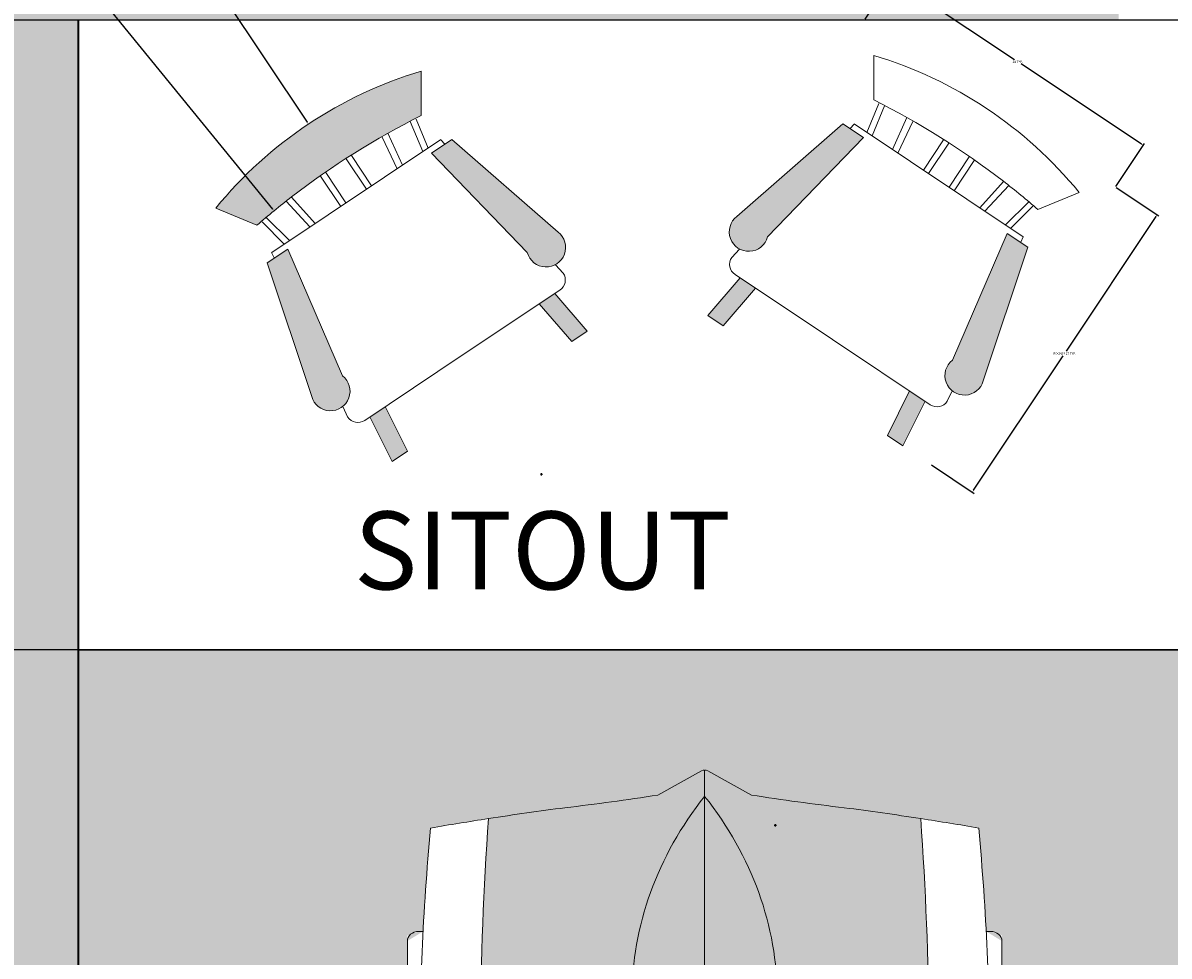
# Model space of a CAD drawing. Units: inches. Extents: x 2549 to 3108, y 1683 to 2362.
# Tile 5 of 30: x 2877 to 2970, y 1861 to 1936. Entities that reach past the tile are written whole.
import ezdxf

# ---------------------------------------------------------------- set-up
doc = ezdxf.new("R2010")
doc.units = ezdxf.units.IN
for name, color, linetype, lineweight in [('A-ANNO-DIMS', 2, 'Continuous', 18), ('A-AREA-IDEN', 7, 'Continuous', 18), ('A-FLOR', 7, 'Continuous', 25), ('A-FURN', 8, 'Continuous', 18), ('A-FURN-PATT', 9, 'Continuous', 13), ('A-WALL', 7, 'Continuous', 35), ('A-WALL-PATT', 89, 'Continuous', 13), ('C-PKNG-VEHI', 8, 'Continuous', 18)]:
    doc.layers.add(name, color=color, linetype=linetype, lineweight=lineweight)
doc.layers.add('C-PKNG-VEHI-PATT', color=251, linetype='Continuous', lineweight=13, true_color=0x636466)
doc.layers.add('C-PVMT-PATT', color=9, linetype='Continuous', lineweight=13, true_color=0xc7c8ca)
doc.styles.get("Standard").update_dxf_attribs({"font": 'arial.ttf'})
doc.dimstyles.get("Standard").update_dxf_attribs({"dimtxt": 0.18, "dimasz": 0.18, "dimexe": 0.18, "dimexo": 0.0625, "dimgap": 0.09, "dimtad": 0, "dimtih": 1, "dimtoh": 1, "dimdec": 4, "dimzin": 0, "dimdsep": 46, "dimtxsty": 'Standard', "dimcen": 0.09, "dimadec": 0, "dimazin": 0, "dimtfac": 1, "dimtdec": 4, "dimtofl": 0, "dimtmove": 0, "dimatfit": 3, "dimfxl": 1, "dimtolj": 1, "dimtzin": 0, "dimarcsym": 0})

# ---------------------------------------------------------------- blocks, each defined once
blk = doc.blocks.new('Chair - Rocking')
for p, q in [((-8, -4.499999999999566), (-10, -1.499999999999566)), ((8, -4.499999999999566), (10, -1.499999999999566)), ((-7.5, -4.499999999999566), (-7, -6.999999999999566)), ((-6.5, -6.999999999999566), (-7.022249999999999, -4.429999999999566)), ((-4.5, -6.999999999999566), (-4.966740000000001, -4.199509999999563)), ((-4, -6.999999999999566), (-4.405320000000003, -4.162719999999573)), ((-1.5, -4.050119999999573), (-1.5, -6.999999999999566)), ((-1, -6.999999999999566), (-1, -4.050119999999573)), ((1, -6.999999999999566), (1, -4.046549999999562)), ((1.5, -4.050119999999573), (1.5, -6.999999999999566)), ((4, -6.999999999999566), (4.401870000000002, -4.186939999999566)), ((4.5, -6.999999999999566), (4.967610000000007, -4.194369999999572)), ((6.5, -6.999999999999566), (7, -4.405699999999562)), ((7.5, -4.499999999999566), (7, -6.999999999999566)), ((-8.234279999999998, -6.999389999999564), (-8.309299999999993, -7.479579999999572)), ((-8.230409999999992, -6.999999999999566), (8.23915000000001, -6.999999999999566)), ((8.31071, -7.488539999999566), (8.234490000000008, -7.00072999999957)), ((-9, -7.499999999999566), (-12, -18.49998999999956)), ((-7, -7.499999999999566), (-9, -7.499999999999566)), ((-9, -18.49998999999956), (-7, -7.499999999999566)), ((7, -7.499999999999566), (9, -7.499999999999566)), ((9, -18.49998999999956), (7, -7.499999999999566)), ((9, -7.499999999999566), (12, -18.49998999999956)), ((-10.36643999999999, -20.64522999999956), (-10.5, -21.49998999999956)), ((10.5, -21.49998999999956), (10.3575, -20.58797999999957)), ((-9, -22.49998999999956), (-9.5, -26.49998999999957)), ((0, -22.49998999999956), (-9.5, -22.49998999999956)), ((-8, -26.49998999999957), (-7.5, -22.49998999999956)), ((0, -22.49998999999956), (9.5, -22.49998999999956)), ((8, -26.49998999999957), (7.5, -22.49998999999956)), ((9, -22.49998999999956), (9.5, -26.49998999999957)), ((-9.5, -26.49998999999957), (-8, -26.49998999999957)), ((9.5, -26.49998999999957), (8, -26.49998999999957))]:
    blk.add_line(p, q)
for centre, radius, start, end in [((0, -34.08332999999957), 34.08332999999957, 72.93847000000062, 107.0614999999994), ((0, -68.25003999999957), 64.24999999999989, 93.92211000000036, 97.15266999999992), ((0, -68.25003999999957), 64.24999999999966, 82.84733000000008, 93.92211000000036), ((-10.5, -18.99998999999956), 1.581138999999956, 161.5650999999866, 18.43495000000615), ((10.5, -18.99998999999956), 1.581138999999949, 161.5650999999865, 18.43495000000615), ((-9.5, -21.49998999999956), 1, 180, 270), ((9.5, -21.49998999999956), 1, 270, 0)]:
    blk.add_arc(centre, radius, start, end)
blk = doc.blocks.new('*U11')
for p, q in [((46.55368679439944, 38.88847654282876), (22.35054758993934, 38.88847654282876)), ((21.10406751471477, 37.40863046792069), (21.10406751471477, 36.83230215753705)), ((3.266462181856987, 6.128290093440767), (0.1022408397004821, 0.4060708604429806)), ((-4.43e-14, -2.558e-13), (51.68362801571248, -2.558e-13)), ((0.1022408397004821, -0.4060708604432933), (3.266462181856987, -6.128290093441194)), ((21.10406751471477, -37.4086304679212), (21.10406751471477, -36.83230215753756)), ((46.55368679439944, -38.88847654282927), (22.35054758993934, -38.88847654282927))]:
    blk.add_line(p, q)
for centre, major_axis, ratio, start_param, end_param in [((22.35054758993934, 37.40863046792072), (2.08e-14, -1.479846074908118), 0.842303869543976, 3.141592653589776, 4.712388980384677), ((41.19115208863305, -490.8631038926156), (1.294e-13, 528.2339998381949), 0.8423038695439741, 0.0028100083536837, 0.0755983031096952), ((266.0300214172791, -27.52442688366631), (1.966072e-10, 313.3077612809058), 0.8423038695435284, 1.367075990158062, 1.391760499156098), ((37.47375371777758, -593.9621830607928), (6.21e-14, -623.32820996736), 0.8423038695439826, 3.09604606856106, 3.200911180495224), ((259.1750197310735, -27.52442688366614), (1.506617e-10, -305.3028914627677), 0.8423038695443789, 4.528606069860317, 4.561837674556238), ((-204.4946649195746, 52.39684969293512), (4.12053e-11, -250.9602162198571), 0.8423038695441164, 1.385369446298923, 1.434372047871027), ((29.77279020470884, -46.66302566589627), (5.12e-14, 56.16885904951626), 0.842303869543976, 7e-16, 0.5903187773915901), ((0.6232400376122422, -1.421e-13), (1e-16, -0.7399230374541245), 0.842303869543842, 4.131459131953847, 5.293318828815531), ((29.77279020470884, 46.66302566589578), (4.004e-13, 56.16885904951626), 0.8423038695439734, 2.55127387619821, 3.141592653589801), ((-204.4946649195746, -52.39684969293552), (4.02945e-11, 250.9602162198562), 0.8423038695441192, -1.43437204787103, -1.385369446298926), ((259.1750197310694, 27.52442688365929), (1.08535e-11, 305.3028914629043), 0.8423038695439974, 1.721347632622872, 1.754579237318777), ((266.0300214172791, 27.52442688366566), (8.75241e-11, 313.3077612806533), 0.8423038695441819, 1.749832154434603, 1.774516663432659), ((37.47375371777847, 593.9621830607904), (1.1693e-12, -623.3282099673584), 0.8423038695439528, -0.0593185269054384, 0.0455465850287298), ((41.19115208863322, 490.8631038926152), (1.37757e-11, -528.2339998381949), 0.8423038695440652, -0.0755983031097181, -0.0028100083537155), ((22.35054758993934, -37.40863046792117), (2.2e-14, 1.479846074908118), 0.8423038695439758, 1.570796326794908, 3.14159265358981)]:
    blk.add_ellipse(centre, major_axis=major_axis, ratio=ratio, start_param=start_param, end_param=end_param)
blk = doc.blocks.new('*D18')
at = {"layer": 'A-ANNO-DIMS', "color": 0, "lineweight": -2, "transparency": 16777216}
for p, q in [((2965.738053794754, 1922.969530017139), (2969.205622138272, 1920.657817788128)), ((2968.95600704997, 1920.607894770468), (2961.689490544522, 1909.708120012294)), ((2954.178799414243, 1898.442083316875), (2961.445315919692, 1909.341858075049)), ((2950.761154088386, 1900.504180457586), (2954.228722431904, 1898.192468228574))]:
    blk.add_line(p, q, dxfattribs=at)
at = {"layer": 'A-ANNO-DIMS', "color": 0, "transparency": 16777216}
for points in [[(2968.931045541141, 1920.624535776354), (2968.980968558801, 1920.591253764581), (2969.05585308529, 1920.757663823448)], [(2954.153837905413, 1898.458724322762), (2954.203760923073, 1898.425442310989), (2954.078953378923, 1898.292314263895)]]:
    blk.add_solid(points, dxfattribs=at)
at = {"layer": 'Defpoints', "color": 0, "transparency": 16777216}
for p in [(2965.686050651358, 1923.004198779404), (2969.05585308529, 1920.757663823448), (2950.70915094499, 1900.53884921985)]:
    blk.add_point(p, dxfattribs=at)
at = {"layer": 'A-ANNO-DIMS', "color": 0, "transparency": 16777216, "insert": (2961.567403232107, 1909.524989043672), "char_height": 0.18, "attachment_point": 5}
blk.add_mtext('\\A1;ROCKER 27 TYP.', dxfattribs=at)
blk = doc.blocks.new('*D19')
at = {"layer": 'A-ANNO-DIMS', "color": 0, "lineweight": -2, "transparency": 16777216}
for p, q in [((2945.38949374051, 1936.610352371541), (2947.701205969521, 1940.077920715058)), ((2947.751128987182, 1939.828305626757), (2957.49632815957, 1933.331506178498)), ((2967.782816554333, 1926.473847248657), (2958.037617381944, 1932.970646696915)), ((2965.720719413623, 1923.0562019228), (2968.032431642634, 1926.523770266317))]:
    blk.add_line(p, q, dxfattribs=at)
at = {"layer": 'A-ANNO-DIMS', "color": 0, "transparency": 16777216}
for points in [[(2947.767769993069, 1939.853267135587), (2947.734487981295, 1939.803344117927), (2947.6013599342, 1939.928151662078)], [(2967.799457560219, 1926.498808757487), (2967.766175548446, 1926.448885739827), (2967.932585607313, 1926.374001213336)]]:
    blk.add_solid(points, dxfattribs=at)
at = {"layer": 'Defpoints', "color": 0, "transparency": 16777216}
for p in [(2947.6013599342, 1939.928151662078), (2945.354824978246, 1936.558349228145), (2965.686050651358, 1923.004198779404)]:
    blk.add_point(p, dxfattribs=at)
at = {"layer": 'A-ANNO-DIMS', "color": 0, "transparency": 16777216, "insert": (2957.766972770757, 1933.151076437707), "char_height": 0.18, "attachment_point": 5}
blk.add_mtext('\\A1;24 TYP.', dxfattribs=at)
blk = doc.blocks.new('*D46')
at = {"layer": 'A-ANNO-DIMS', "color": 0, "lineweight": -2, "transparency": 16777216}
for p, q in [((2812.642666, 2140.461244), (2812.642666, 1683.443744)), ((3034.642666, 2134.461244), (3034.642666, 1683.443744)), ((2812.822666, 1683.623744), (2923.35320488131, 1683.623744)), ((3034.462666, 1683.623744), (2923.932127118691, 1683.623744))]:
    blk.add_line(p, q, dxfattribs=at)
at = {"layer": 'A-ANNO-DIMS', "color": 0, "transparency": 16777216}
for points in [[(2812.822666, 1683.653744), (2812.822666, 1683.593744), (2812.642666, 1683.623744)], [(3034.462666, 1683.653744), (3034.462666, 1683.593744), (3034.642666, 1683.623744)]]:
    blk.add_solid(points, dxfattribs=at)
at = {"layer": 'Defpoints', "color": 0, "transparency": 16777216}
for p in [(2812.642666, 2140.523744), (3034.642666, 2134.523744), (3034.642666, 1683.623744)]:
    blk.add_point(p, dxfattribs=at)
at = {"layer": 'A-ANNO-DIMS', "color": 0, "transparency": 16777216, "insert": (2923.642666000001, 1683.623744), "char_height": 0.18, "attachment_point": 5}
blk.add_mtext('\\A1;222', dxfattribs=at)
blk = doc.blocks.new('*D56')
at = {"layer": 'A-ANNO-DIMS', "color": 0, "lineweight": -2, "transparency": 16777216}
for p, q in [((3043.580166000001, 1936.523744000001), (2549.424763000002, 1936.523744000001)), ((2549.604763000002, 1936.343744000001), (2549.604763000002, 1911.205647137791)), ((2549.604763000002, 1885.703744000001), (2549.604763000002, 1910.841840862211)), ((3043.580166000001, 1885.523744000001), (2549.424763000002, 1885.523744000001))]:
    blk.add_line(p, q, dxfattribs=at)
at = {"layer": 'A-ANNO-DIMS', "color": 0, "transparency": 16777216}
for points in [[(2549.574763000002, 1936.343744000001), (2549.634763000002, 1936.343744000001), (2549.604763000002, 1936.523744000001)], [(2549.574763000002, 1885.703744000001), (2549.634763000002, 1885.703744000001), (2549.604763000002, 1885.523744000001)]]:
    blk.add_solid(points, dxfattribs=at)
at = {"layer": 'Defpoints', "color": 0, "transparency": 16777216}
for p in [(2549.604763000002, 1936.523744000001), (3043.642666000001, 1936.523744000001), (3043.642666000001, 1885.523744000001)]:
    blk.add_point(p, dxfattribs=at)
at = {"layer": 'A-ANNO-DIMS', "color": 0, "transparency": 16777216, "insert": (2549.604763000002, 1911.023743999999), "char_height": 0.18, "attachment_point": 5}
blk.add_mtext('\\A1;51', dxfattribs=at)
blk = doc.blocks.new('*D66')
at = {"layer": 'A-ANNO-DIMS', "color": 0, "lineweight": -2, "transparency": 16777216}
for p, q in [((2872.93362808891, 1950.941863936075), (2873.11362808891, 1950.941863936074)), ((2873.11362808891, 1950.941863936074), (2897.37882396306, 1921.218856531219)), ((2938.034368999999, 1871.308682999998), (2938.214368999999, 1871.308682999999)), ((2938.124368999999, 1871.218682999999), (2938.124369, 1871.398682999999))]:
    blk.add_line(p, q, dxfattribs=at)
at = {"layer": 'A-ANNO-DIMS', "color": 0, "transparency": 16777216}
blk.add_solid([(2897.402063218263, 1921.237828537375), (2897.355584707857, 1921.199884525062), (2897.492655999999, 1921.079420999999)], dxfattribs=at)
at = {"layer": 'Defpoints', "color": 0, "transparency": 16777216}
for p in [(2897.492655999999, 1921.079420999999), (2938.124369, 1871.308682999999)]:
    blk.add_point(p, dxfattribs=at)
at = {"layer": 'A-ANNO-DIMS', "color": 0, "transparency": 16777216, "insert": (2872.258198348119, 1950.941863936074), "char_height": 0.18, "attachment_point": 5}
blk.add_mtext('\\A1;2X R64.25', dxfattribs=at)
blk = doc.blocks.new('*D67')
at = {"layer": 'A-ANNO-DIMS', "color": 0, "lineweight": -2, "transparency": 16777216}
for p, q in [((2888.742267019754, 1945.111459470369), (2888.922267019754, 1945.111459470369)), ((2888.922267019754, 1945.111459470369), (2900.166103391877, 1928.245844671111)), ((2919.082088, 1899.737104), (2919.262088, 1899.737104)), ((2919.172088000001, 1899.647104000001), (2919.172088, 1899.827104))]:
    blk.add_line(p, q, dxfattribs=at)
at = {"layer": 'A-ANNO-DIMS', "color": 0, "transparency": 16777216}
blk.add_solid([(2900.191064837062, 1928.262485772465), (2900.141141946692, 1928.229203569756), (2900.265950000001, 1928.096076)], dxfattribs=at)
at = {"layer": 'Defpoints', "color": 0, "transparency": 16777216}
for p in [(2900.265950000001, 1928.096076), (2919.172088, 1899.737104)]:
    blk.add_point(p, dxfattribs=at)
at = {"layer": 'A-ANNO-DIMS', "color": 0, "transparency": 16777216, "insert": (2888.262246555907, 1945.111459470368), "char_height": 0.18, "attachment_point": 5}
blk.add_mtext('\\A1;R34.08', dxfattribs=at)

msp = doc.modelspace()

# ---------------------------------------------------------------- hatches: boundary and pattern name
at = {"layer": 'A-FURN-PATT', "transparency": 33554567}
h = msp.add_hatch(color=256, dxfattribs=at)
h.dxf.hatch_style = 1
h.paths.add_polyline_path([(2708.714672869869, 2271.673744486262), (2675.281339536536, 2271.673744486262), (2675.281339536536, 2262.040411152929), (2708.714672869869, 2262.040411152929)])
h.paths.add_polyline_path([(2980.824596989089, 2271.673744486262), (2947.391263655756, 2271.673744486262), (2947.391263655756, 2262.040411152929), (2980.824596989089, 2262.040411152929)])
h.paths.add_polyline_path([(2748.849609196547, 2101.638310911291), (2798.147998217048, 2101.638310911291), (2798.147998217048, 2111.424826549233), (2748.849609196547, 2111.424826549233)], flags=9)
h.paths.add_polyline_path([(2685.208067619545, 2101.488974631509), (2719.325307162104, 2101.488974631509), (2719.325307162104, 2111.281945754699), (2685.208067619545, 2111.281945754699)], flags=9)
h.paths.add_polyline_path([(2814.685179139321, 1907.132804880864), (2847.838399551318, 1907.132804880864), (2847.838399551318, 1916.925776004054), (2814.685179139321, 1916.925776004054)], flags=9)
h.paths.add_polyline_path([(2814.390575309562, 1835.586397562281), (2848.017197973174, 1835.586397562281), (2848.017197973174, 1845.379368685471), (2814.390575309562, 1845.379368685471)], flags=9)
h.paths.add_polyline_path([(2800.524456569608, 1759.167447237475), (2853.743476964851, 1759.167447237475), (2853.743476964851, 1768.953962875417), (2800.524456569608, 1768.953962875417)], flags=9)
h.paths.add_polyline_path([(2972.461062245805, 1807.33049128039), (3015.394342810494, 1807.33049128039), (3015.394342810494, 1817.117006918332), (2972.461062245805, 1817.117006918332)], flags=9)
h.paths.add_polyline_path([(2902.332650472062, 1888.673085326325), (2937.913133337796, 1888.673085326325), (2937.913133337796, 1898.466056449515), (2902.332650472062, 1898.466056449515)], flags=9)
h.paths.add_polyline_path([(2712.17793111998, 1878.903902566108), (2754.125674269943, 1878.903902566108), (2754.125674269943, 1888.69041820405), (2712.17793111998, 1888.69041820405)], flags=9)
h.paths.add_polyline_path([(2614.005606808349, 2012.811964980989), (2650.025062671036, 2012.811964980989), (2650.025062671036, 2022.437093487698), (2614.005606808349, 2022.437093487698)], flags=9)
h.paths.add_polyline_path([(2713.312922761346, 2003.164487508756), (2747.423706818656, 2003.164487508756), (2747.423706818656, 2012.951003146698), (2713.312922761346, 2012.951003146698)], flags=9)
h.paths.add_polyline_path([(2950.137937233872, 2001.693439459313), (2982.299164745893, 2001.693439459313), (2982.299164745893, 2011.479955097255), (2950.137937233872, 2011.479955097255)], flags=9)
h.paths.add_polyline_path([(2940.863994744806, 2238.553674899427), (2997.506574150595, 2238.553674899427), (2997.506574150595, 2248.346646022617), (2940.863994744806, 2248.346646022617)], flags=9)
h.paths.add_polyline_path([(2821.545730132573, 2202.834824551463), (2855.662969675132, 2202.834824551463), (2855.662969675132, 2212.627795674654), (2821.545730132573, 2212.627795674654)], flags=9)
h.paths.add_polyline_path([(2661.802564922812, 2238.624912952816), (2718.445144328601, 2238.624912952816), (2718.445144328601, 2248.417884076006), (2661.802564922812, 2248.417884076006)], flags=9)
h = msp.add_hatch(color=256, dxfattribs=at)
h.dxf.hatch_style = 1
h.paths.add_polyline_path([(2906.506430286822, 1905.214773716388), (2905.258354845315, 1904.38272342205), (2907.061130483047, 1900.777172146586), (2908.309205924554, 1901.609222440924)])
h.paths.add_polyline_path([(2936.521961741216, 1914.804377056317), (2935.27388629971, 1915.636427350655), (2932.63906036764, 1912.585576271416), (2933.887135809147, 1911.753525977078)])
h.paths.add_polyline_path([(2950.250791597791, 1905.651823818601), (2949.002716156284, 1906.483874112939), (2947.199940518553, 1902.878322837475), (2948.448015960059, 1902.046272543137)])
h.paths.add_polyline_path([(2958.571288994167, 1918.132569913166), (2956.907188405492, 1919.241970305616), (2952.469592522951, 1908.980025320303, 1.387427444474919), (2954.965744234361, 1907.315927313246)])
h.paths.add_polyline_path([(2945.258484284762, 1927.007773052769), (2943.594383696085, 1928.11717344522), (2934.996538511474, 1920.62873112851, 1.38742744447752), (2937.492687330065, 1918.964628782227)])
h.paths.add_polyline_path([(2748.849609196547, 2101.638310911291), (2798.147998217048, 2101.638310911291), (2798.147998217048, 2111.424826549233), (2748.849609196547, 2111.424826549233)], flags=9)
h.paths.add_polyline_path([(2685.208067619545, 2101.488974631509), (2719.325307162104, 2101.488974631509), (2719.325307162104, 2111.281945754699), (2685.208067619545, 2111.281945754699)], flags=9)
h.paths.add_polyline_path([(2814.685179139321, 1907.132804880864), (2847.838399551318, 1907.132804880864), (2847.838399551318, 1916.925776004054), (2814.685179139321, 1916.925776004054)], flags=9)
h.paths.add_polyline_path([(2814.390575309562, 1835.586397562281), (2848.017197973174, 1835.586397562281), (2848.017197973174, 1845.379368685471), (2814.390575309562, 1845.379368685471)], flags=9)
h.paths.add_polyline_path([(2800.524456569608, 1759.167447237475), (2853.743476964851, 1759.167447237475), (2853.743476964851, 1768.953962875417), (2800.524456569608, 1768.953962875417)], flags=9)
h.paths.add_polyline_path([(2972.461062245805, 1807.33049128039), (3015.394342810494, 1807.33049128039), (3015.394342810494, 1817.117006918332), (2972.461062245805, 1817.117006918332)], flags=9)
h.paths.add_polyline_path([(2902.332650472062, 1888.673085326325), (2937.913133337796, 1888.673085326325), (2937.913133337796, 1898.466056449515), (2902.332650472062, 1898.466056449515)], flags=9)
h.paths.add_polyline_path([(2712.17793111998, 1878.903902566108), (2754.125674269943, 1878.903902566108), (2754.125674269943, 1888.69041820405), (2712.17793111998, 1888.69041820405)], flags=9)
h.paths.add_polyline_path([(2614.005606808349, 2012.811964980989), (2650.025062671036, 2012.811964980989), (2650.025062671036, 2022.437093487698), (2614.005606808349, 2022.437093487698)], flags=9)
h.paths.add_polyline_path([(2713.312922761346, 2003.164487508756), (2747.423706818656, 2003.164487508756), (2747.423706818656, 2012.951003146698), (2713.312922761346, 2012.951003146698)], flags=9)
h.paths.add_polyline_path([(2950.137937233872, 2001.693439459313), (2982.299164745893, 2001.693439459313), (2982.299164745893, 2011.479955097255), (2950.137937233872, 2011.479955097255)], flags=9)
h.paths.add_polyline_path([(2940.863994744806, 2238.553674899427), (2997.506574150595, 2238.553674899427), (2997.506574150595, 2248.346646022617), (2940.863994744806, 2248.346646022617)], flags=9)
h.paths.add_polyline_path([(2821.545730132573, 2202.834824551463), (2855.662969675132, 2202.834824551463), (2855.662969675132, 2212.627795674654), (2821.545730132573, 2212.627795674654)], flags=9)
h.paths.add_polyline_path([(2661.802564922812, 2238.624912952816), (2718.445144328601, 2238.624912952816), (2718.445144328601, 2248.417884076006), (2661.802564922812, 2248.417884076006)], flags=9)
h = msp.add_hatch(color=256, dxfattribs=at)
h.dxf.hatch_style = 1
h.paths.add_polyline_path([(2911.91476274702, 1926.848073048669), (2910.250662158345, 1925.738672656219), (2918.016459113041, 1917.695528385677, 1.387427444473759), (2920.512607931638, 1919.359630731954)])
h.paths.add_polyline_path([(2898.601958037615, 1917.972869909066), (2896.937857448939, 1916.863469516615), (2900.543402208745, 1906.046826916695, 1.387427444474816), (2903.039553920154, 1907.710924923753)])
h.paths.add_polyline_path([(2909.418611864007, 1928.789479372818), (2909.418611864007, 1932.395074857819, 0.1500000140127385), (2892.777606118574, 1921.301071027532), (2896.105848104729, 1919.9143035333, -0.0140968088762487), (2898.911724151526, 1922.20495918066, -0.0483603895502414)])
h.paths.add_polyline_path([(2920.235260143396, 1914.367326954105), (2918.98718470189, 1913.535276659767), (2921.622010633959, 1910.484425580528), (2922.870086075466, 1911.316475874866)])
at = {"layer": 'A-WALL-PATT'}
h = msp.add_hatch(color=256, dxfattribs=at)
h.dxf.hatch_style = 1
h.paths.add_polyline_path([(2638.642666391656, 2272.523744486262), (3034.642666391656, 2272.523744486262), (3034.642666391656, 1936.523744486262), (3043.642666391656, 1936.523744486262), (3043.642666391656, 2281.523744486262), (2629.642666391656, 2281.523744486262), (2629.642666391656, 2074.523744486262), (2812.642666391655, 2074.523744486262), (2812.642666391655, 2140.523744486262), (2785.717675498527, 2140.523744486262), (2785.717675498527, 2134.523744486262), (2806.642666391656, 2134.523744486262), (2806.642666391656, 2080.523744486262), (2638.642666391656, 2080.523744486262)])
h.paths.add_polyline_path([(2638.642666391656, 1972.523744486262), (2662.642666391656, 1972.523744486262), (2662.642666391656, 2041.055679691546), (2653.642666391655, 2041.055679691546), (2653.642666391656, 1978.523744486262), (2629.642666391656, 1978.523744486262), (2629.642666391656, 1795.523744486262), (2662.642666391656, 1795.523744486262), (2881.642666391656, 1795.523744486262), (2881.642666391656, 1936.523744486262), (2965.935139880862, 1936.523744486262), (2965.935139880862, 1974.543933838007), (2959.935139880861, 1974.543933838007), (2959.935139880861, 1945.523744486262), (2881.642666391656, 1945.523744486262), (2872.642666391655, 1945.523744486262), (2872.642666391655, 1804.523744486262), (2662.642666391656, 1804.523744486262), (2638.642666391656, 1804.523744486262)])
at = {"layer": 'C-PKNG-VEHI-PATT'}
h = msp.add_hatch(color=256, dxfattribs=at)
h.dxf.hatch_style = 1
edge = h.paths.add_edge_path()
edge.add_ellipse((2935.725796552836, 1791.96404850691), major_axis=(-50.6600031146233, 6.78e-13), ratio=0.8423038695439883, start_angle=248.1650462032912, end_angle=265.7225790369452)
edge.add_line((2938.911028887629, 1834.550737322417), (2925.865275339109, 1834.550737322417))
edge.add_ellipse((2929.050507673901, 1791.964048506909), major_axis=(50.66000311462998, 7.2698e-12), ratio=0.8423038695438956, start_angle=94.27742096304536, end_angle=111.8349537966996)
edge.add_line((2912.850791291541, 1832.394679033669), (2914.204376096751, 1822.249450253823))
edge.add_ellipse((2930.653832861207, 1783.102276333115), major_axis=(-49.30143828149606, 1.1087e-12), ratio=0.8423038695440098, start_angle=-85.12993040286318, end_angle=-67.20808512241217, ccw=False)
edge.add_line((2927.124659327709, 1824.522535937876), (2937.65164489903, 1824.522535937876))
edge.add_ellipse((2934.122471365533, 1783.102276333124), major_axis=(49.30143828148681, 7.803e-13), ratio=0.8423038695439693, start_angle=67.20808512240922, end_angle=85.12993040286312, ccw=False)
edge.add_line((2950.571928129987, 1822.249450253823), (2951.925512935197, 1832.394679033669))
edge = h.paths.add_edge_path()
edge.add_ellipse((2903.479330909537, 1857.335124490177), major_axis=(-34.79790434319148, 3.2087e-12), ratio=0.8423038695440206, start_angle=180.0000000000052, end_angle=209.4385695979841)
edge.add_ellipse((2961.296973317201, 1857.335124490177), major_axis=(34.79790434319149, 1.2616e-12), ratio=0.8423038695439669, start_angle=150.5614304020187, end_angle=179.9999999999979)
edge.add_line((2926.49906897401, 1857.335124490177), (2926.49906897401, 1843.76085484809))
edge.add_ellipse((2924.125124210826, 1844.314306179491), major_axis=(-0.2209272451118966, 3.927824345135514), ratio=0.6038335755719296, start_angle=89.00201427502537, end_angle=253.65740804569998, ccw=False)
edge.add_line((2921.751179447642, 1844.222223668088), (2921.751179447642, 1853.39746861696))
edge.add_line((2921.751179447642, 1853.39746861696), (2925.26903797625, 1855.848425453852))
edge.add_ellipse((2925.478177919096, 1855.493055533625), major_axis=(0.4583993962922678, 2.303e-12), ratio=0.8423038695418179, start_angle=89.9999999997122, end_angle=134.4802108822853, ccw=False)
edge.add_line((2925.478177919095, 1855.879167118917), (2926.49906897401, 1855.879167118917))
edge.add_line((2926.49906897401, 1855.879167118917), (2926.49906897401, 1857.335124490177))
edge.add_ellipse((2961.296973317201, 1857.335124490177), major_axis=(34.79790434319149, 1.2616e-12), ratio=0.8423038695439669, start_angle=150.5614304020187, end_angle=179.999999999998, ccw=False)
edge.add_line((2932.388152113369, 1873.650056952746), (2932.388152113369, 1875.780055063896))
edge.add_ellipse((2932.388152113369, 1875.393943478604), major_axis=(0.4583993962904624, 1e-16), ratio=0.8423038695446395, start_angle=89.99999999999999, end_angle=127.9331304598429)
edge.add_line((2932.136581844764, 1875.716714504374), (2928.591534983032, 1873.756406364807))
edge.add_ellipse((2899.927094610101, 2002.469218934773), major_axis=(155.4756451483881, 9.82606e-11), ratio=0.842303869543439, start_angle=-80.74343399283458, end_angle=-77.44506735589891, ccw=False)
edge.add_ellipse((2949.440169726089, 1715.215149574257), major_axis=(-189.1421864819335, 9.35831e-11), ratio=0.8423038695443681, start_angle=-79.79046100282835, end_angle=-77.55537270652765)
edge.add_ellipse((3300.361430890526, 1852.564199885104), major_axis=(-386.1662101011402, 3.282e-12), ratio=0.8423038695438535, start_angle=-2.863714607837213, end_angle=2.198540565955553)
edge.add_ellipse((2929.050507673902, 1792.515918881865), major_axis=(-55.61920468847034, 9.624e-12), ratio=0.842303869544118, start_angle=-85.91758930883981, end_angle=-72.28004677724027, ccw=False)
edge.add_line((2925.712863234435, 1839.27976237288), (2939.063440992303, 1839.27976237288))
edge.add_ellipse((2935.725796552836, 1792.515918881865), major_axis=(55.61920468846977, 1.19088e-11), ratio=0.8423038695441256, start_angle=72.28004677723749, end_angle=85.91758930883759, ccw=False)
edge.add_ellipse((2564.414873336211, 1852.564199885105), major_axis=(-386.166210101141, 7.3121e-12), ratio=0.8423038695442235, start_angle=177.8014594340458, end_angle=182.8637146078386)
edge.add_ellipse((2915.336134500645, 1715.215149574254), major_axis=(189.1421864814668, 5.425418e-10), ratio=0.8423038695464061, start_angle=77.5553727063904, end_angle=79.79046100269107)
edge.add_ellipse((2964.849209616638, 2002.469218934773), major_axis=(-155.4756451483861, 9.70869e-11), ratio=0.8423038695434499, start_angle=77.44506735589852, end_angle=80.74343399283418, ccw=False)
edge.add_line((2936.184769243706, 1873.756406364807), (2932.639722381973, 1875.716714504375))
edge.add_ellipse((2932.388152113369, 1875.393943478604), major_axis=(0.4583993962904624, 1e-16), ratio=0.8423038695446395, start_angle=52.06686954015704, end_angle=89.99999999999999)
edge.add_line((2932.388152113369, 1875.780055063896), (2932.388152113369, 1873.650056952746))
edge.add_ellipse((2903.479330909537, 1857.335124490177), major_axis=(-34.79790434319148, 3.2087e-12), ratio=0.8423038695440206, start_angle=180.0000000000053, end_angle=209.4385695979841, ccw=False)
edge.add_line((2938.277235252728, 1857.335124490177), (2938.277235252728, 1855.879167118917))
edge.add_line((2938.277235252728, 1855.879167118917), (2939.405880844674, 1855.879167118917))
edge.add_ellipse((2939.298126307642, 1855.493055533625), major_axis=(-0.4583993962922676, 2.3028e-12), ratio=0.8423038695418185, start_angle=225.5197891177147, end_angle=270.00000000028786, ccw=False)
edge.add_line((2939.590297193029, 1855.790576266728), (2943.025124779096, 1853.39746861696))
edge.add_line((2943.025124779096, 1853.39746861696), (2943.025124779096, 1844.222223668088))
edge.add_ellipse((2940.651180015912, 1844.314306179491), major_axis=(0.2209272451118966, 3.927824345135514), ratio=0.6038335755719296, start_angle=106.3425919543001, end_angle=270.9979857249746, ccw=False)
edge.add_line((2938.277235252728, 1843.76085484809), (2938.277235252728, 1857.335124490177))
edge = h.paths.add_edge_path()
edge.add_ellipse((2932.388152113369, 1865.19731394932), major_axis=(91.08099646002908, 7.134e-13), ratio=0.8423038695439837, start_angle=256.4018653097688, end_angle=283.5981346902299, ccw=False)
edge.add_line((2914.204376096751, 1790.023884530285), (2914.204376096751, 1778.36217788565))
edge.add_ellipse((2932.388152113369, 1853.535607304685), major_axis=(91.08099646002908, 7.134e-13), ratio=0.8423038695439837, start_angle=256.4018653097688, end_angle=283.5981346902299)
edge.add_line((2950.571928129987, 1778.36217788565), (2950.571928129987, 1790.023884530285))
edge = h.paths.add_edge_path()
edge.add_ellipse((2948.738330544823, 1772.31452600415), major_axis=(1.833597585163715, 1.1861e-12), ratio=0.8423038695440299, start_angle=-3.70558e-11, end_angle=89.99999999996297)
edge.add_line((2948.738330544824, 1773.85897234532), (2916.037973681915, 1773.858972345321))
edge.add_ellipse((2916.037973681915, 1772.314526004151), major_axis=(1.833597585163716, 6.788e-13), ratio=0.84230386954403, start_angle=89.9999999999788, end_angle=179.9999999999787)
edge.add_line((2914.204376096751, 1772.314526004151), (2914.204376096751, 1760.255799913309))
edge.add_line((2914.204376096751, 1760.255799913309), (2950.571928129987, 1760.255799913308))
edge.add_line((2950.571928129987, 1760.255799913308), (2950.571928129987, 1772.31452600415))
h.paths.add_polyline_path([(2748.849609196547, 2101.638310911291), (2798.147998217048, 2101.638310911291), (2798.147998217048, 2111.424826549233), (2748.849609196547, 2111.424826549233)], flags=9)
h.paths.add_polyline_path([(2685.208067619545, 2101.488974631509), (2719.325307162104, 2101.488974631509), (2719.325307162104, 2111.281945754699), (2685.208067619545, 2111.281945754699)], flags=9)
h.paths.add_polyline_path([(2814.685179139321, 1907.132804880864), (2847.838399551318, 1907.132804880864), (2847.838399551318, 1916.925776004054), (2814.685179139321, 1916.925776004054)], flags=9)
h.paths.add_polyline_path([(2814.390575309562, 1835.586397562281), (2848.017197973174, 1835.586397562281), (2848.017197973174, 1845.379368685471), (2814.390575309562, 1845.379368685471)], flags=9)
h.paths.add_polyline_path([(2800.524456569608, 1759.167447237475), (2853.743476964851, 1759.167447237475), (2853.743476964851, 1768.953962875417), (2800.524456569608, 1768.953962875417)], flags=9)
h.paths.add_polyline_path([(2972.461062245805, 1807.33049128039), (3015.394342810494, 1807.33049128039), (3015.394342810494, 1817.117006918332), (2972.461062245805, 1817.117006918332)], flags=9)
h.paths.add_polyline_path([(2902.332650472062, 1888.673085326325), (2937.913133337796, 1888.673085326325), (2937.913133337796, 1898.466056449515), (2902.332650472062, 1898.466056449515)], flags=9)
h.paths.add_polyline_path([(2712.17793111998, 1878.903902566108), (2754.125674269943, 1878.903902566108), (2754.125674269943, 1888.69041820405), (2712.17793111998, 1888.69041820405)], flags=9)
h.paths.add_polyline_path([(2614.005606808349, 2012.811964980989), (2650.025062671036, 2012.811964980989), (2650.025062671036, 2022.437093487698), (2614.005606808349, 2022.437093487698)], flags=9)
h.paths.add_polyline_path([(2713.312922761346, 2003.164487508756), (2747.423706818656, 2003.164487508756), (2747.423706818656, 2012.951003146698), (2713.312922761346, 2012.951003146698)], flags=9)
h.paths.add_polyline_path([(2950.137937233872, 2001.693439459313), (2982.299164745893, 2001.693439459313), (2982.299164745893, 2011.479955097255), (2950.137937233872, 2011.479955097255)], flags=9)
h.paths.add_polyline_path([(2940.863994744806, 2238.553674899427), (2997.506574150595, 2238.553674899427), (2997.506574150595, 2248.346646022617), (2940.863994744806, 2248.346646022617)], flags=9)
h.paths.add_polyline_path([(2821.545730132573, 2202.834824551463), (2855.662969675132, 2202.834824551463), (2855.662969675132, 2212.627795674654), (2821.545730132573, 2212.627795674654)], flags=9)
h.paths.add_polyline_path([(2661.802564922812, 2238.624912952816), (2718.445144328601, 2238.624912952816), (2718.445144328601, 2248.417884076006), (2661.802564922812, 2248.417884076006)], flags=9)
at = {"layer": 'C-PVMT-PATT'}
h = msp.add_hatch(color=256, dxfattribs=at)
h.dxf.hatch_style = 1
h.paths.add_polyline_path([(3067.642666391656, 2305.523744486262), (2605.642666391656, 2305.523744486262), (2605.642666391656, 2074.523744486262), (2629.642666391656, 2074.523744486262), (2629.642666391656, 2281.523744486262), (3043.642666391656, 2281.523744486262), (3043.642666391656, 1885.523744486263), (3043.642666391656, 1872.874514030248), (3031.167181590035, 1872.874514030248), (3031.167181590035, 1862.573058982011), (2995.805391311171, 1862.573058982011), (2995.805391311171, 1872.874514030248), (2983.175155144805, 1872.874514030248), (2983.175155144805, 1885.523744486262), (2881.642666391656, 1885.523744486263), (2881.642666391656, 1795.523744486262), (2751.09773888662, 1795.523744486262), (2751.09773888662, 1761.523744486262), (2786.157685455576, 1761.523744486262), (2786.157685455577, 1723.523744486262), (2881.839988255281, 1723.523744486262), (2881.839988255281, 1714.523744486262), (3067.642666391656, 1714.523744486262), (3067.642666391656, 1723.523744486262)])
edge = h.paths.add_edge_path(flags=16)
edge.add_ellipse((2949.440169726093, 1710.96831784248), major_axis=(-194.1013880556022, 3.100242e-10), ratio=0.8423038695451509, start_angle=-77.87403444762441, end_angle=-76.21947101041059, ccw=False)
edge.add_ellipse((2949.440169726089, 1715.215149574257), major_axis=(-189.1421864819335, 9.35831e-11), ratio=0.8423038695443681, start_angle=-79.7904610028283, end_angle=-77.55537270652758, ccw=False)
edge.add_ellipse((2899.927094610101, 2002.469218934773), major_axis=(155.4756451483881, 9.82606e-11), ratio=0.842303869543439, start_angle=-80.74343399283462, end_angle=-77.44506735589897)
edge.add_line((2928.591534983032, 1873.756406364807), (2932.388152113369, 1875.855825569603))
edge.add_line((2932.388152113369, 1875.855825569603), (2936.184769243706, 1873.756406364807))
edge.add_ellipse((2964.849209616638, 2002.469218934773), major_axis=(-155.4756451483861, 9.70869e-11), ratio=0.8423038695434499, start_angle=77.4450673558985, end_angle=80.74343399283416)
edge.add_ellipse((2915.336134500645, 1715.215149574254), major_axis=(189.1421864814668, 5.425418e-10), ratio=0.8423038695464061, start_angle=77.55537270639041, end_angle=79.79046100269102, ccw=False)
edge.add_ellipse((2915.336134500645, 1710.96831784248), major_axis=(-194.1013880561466, 2.794238e-10), ratio=0.8423038695428703, start_angle=256.2194710105847, end_angle=257.8740344477983, ccw=False)
edge.add_ellipse((2628.287132012546, 1850.261185811051), major_axis=(-327.2531525161749, 1.24457e-11), ratio=0.8423038695440036, start_angle=182.1799503136474, end_angle=183.6504275857012, ccw=False)
edge.add_ellipse((2955.563661936079, 1861.933375066942), major_axis=(-0.9167987925820851, 6.203e-13), ratio=0.8423038695438211, start_angle=180.0000000000388, end_angle=270.00000000003877, ccw=False)
edge.add_line((2956.480460728661, 1862.385732927092), (2956.480460728661, 1846.486613953928))
edge.add_ellipse((2955.563661936079, 1846.938971814078), major_axis=(-0.9167987925816303, 6.983e-13), ratio=0.8423038695442389, start_angle=90.0000000000436, end_angle=180.0000000000437, ccw=False)
edge.add_ellipse((-3607.060581297885, 1835.831972437108), major_axis=(-6562.624243233964, 2.000376e-10), ratio=0.8423038695434055, start_angle=179.6161332212093, end_angle=180.0902290885961, ccw=False)
edge.add_ellipse((2955.563661936079, 1791.092611498023), major_axis=(0.9167987925816303, 1.8053e-12), ratio=0.8423038695442389, start_angle=-1.127773430198431e-10, end_angle=89.99999999988711, ccw=False)
edge.add_line((2956.480460728661, 1791.544969358173), (2956.480460728661, 1775.645850385008))
edge.add_ellipse((2955.563661936079, 1776.098208245159), major_axis=(0.9167987925816303, 5.91e-14), ratio=0.8423038695442391, start_angle=269.9999999999963, end_angle=359.9999999999963, ccw=False)
edge.add_ellipse((-3607.060581297885, 1835.831972437108), major_axis=(-6562.624243233964, 2.000376e-10), ratio=0.8423038695434055, start_angle=179.3813568036826, end_angle=179.4717285281838, ccw=False)
edge.add_ellipse((2954.590723441648, 1763.876816393945), major_axis=(-1.375198188872997, 3.586e-13), ratio=0.8423038695436877, start_angle=179.3717627838213, end_angle=248.4647566010281, ccw=False)
edge.add_ellipse((-3607.518980694323, 1835.831972435604), major_axis=(-6564.040927375597, 4.0829067806e-06), ratio=0.8423038626957529, start_angle=179.3534459385899, end_angle=179.371762819423, ccw=False)
edge.add_ellipse((2952.682914207262, 1761.800246254478), major_axis=(3.250281735962, 3.921e-13), ratio=0.8423038695438826, start_angle=-89.99999999994031, end_angle=-0.6465540970884831, ccw=False)
edge.add_line((2952.682914207266, 1759.06252137117), (2912.093390019471, 1759.062521371171))
edge.add_ellipse((2912.093390019478, 1761.800246254481), major_axis=(3.250281735963338, 1.2841e-12), ratio=0.8423038695440954, start_angle=180.6465540970387, end_angle=269.99999999984414, ccw=False)
edge.add_ellipse((9472.295284948175, 1835.831972439052), major_axis=(-6564.040927413921, 8.323842912e-07), ratio=0.8423038709559154, start_angle=0.6282372235086768, end_angle=0.646554104341817, ccw=False)
edge.add_ellipse((2910.185580785089, 1763.876816393947), major_axis=(1.375198188873441, 9.687e-13), ratio=0.8423038695438604, start_angle=111.53524350397811, end_angle=180.6282372161342, ccw=False)
edge.add_ellipse((9471.836885542962, 1835.831972437208), major_axis=(-6562.624243252301, 3.836442e-10), ratio=0.8423038695462286, start_angle=0.5282714718206876, end_angle=0.6465540970643247, ccw=False)
edge.add_ellipse((2909.212642290659, 1776.098208245159), major_axis=(-0.9167987925820851, 6.203e-13), ratio=0.8423038695438211, start_angle=3.8824055081931874e-11, end_angle=90.00000000003882, ccw=False)
edge.add_line((2908.295843498077, 1775.645850385009), (2908.295843498077, 1791.544969358173))
edge.add_ellipse((2909.212642290659, 1791.092611498023), major_axis=(-0.9167987925820851, 4.868e-13), ratio=0.8423038695438213, start_angle=-89.99999999996948, end_angle=3.041122909053229e-11, ccw=False)
edge.add_ellipse((9471.836885542962, 1835.831972437208), major_axis=(-6562.624243252301, 3.836442e-10), ratio=0.8423038695462286, start_angle=-0.09022908858980827, end_angle=0.38386677879560693, ccw=False)
edge.add_ellipse((2909.212642290658, 1846.938971814078), major_axis=(-0.9167987925816306, 1.1661e-12), ratio=0.8423038695442389, start_angle=7.287326297955588e-11, end_angle=90.00000000007287, ccw=False)
edge.add_line((2908.295843498077, 1846.486613953928), (2908.295843498077, 1862.385732927092))
edge.add_ellipse((2909.212642290658, 1861.933375066942), major_axis=(0.9167987925816303, 1.1659e-12), ratio=0.8423038695442391, start_angle=89.99999999992713, end_angle=179.9999999999272, ccw=False)
edge.add_ellipse((3236.489172214191, 1850.261185811051), major_axis=(327.2531525161745, 3.33005e-11), ratio=0.8423038695444386, start_angle=176.3495724142951, end_angle=177.820049686349, ccw=False)
edge = h.paths.add_edge_path(flags=0)
edge.add_ellipse((2903.479330909537, 1857.335124490177), major_axis=(-34.79790434319148, 3.2087e-12), ratio=0.8423038695440206, start_angle=180.0000000000053, end_angle=209.4385695979841, ccw=False)
edge.add_line((2938.277235252728, 1857.335124490177), (2938.277235252728, 1855.879167118917))
edge.add_line((2938.277235252728, 1855.879167118917), (2939.463142736354, 1855.879167118917))
edge.add_line((2939.463142736354, 1855.879167118917), (2943.025124779096, 1853.39746861696))
edge.add_line((2943.025124779096, 1853.39746861696), (2943.025124779096, 1844.222223668088))
edge.add_ellipse((2940.651180015912, 1844.314306179491), major_axis=(0.2209272451118966, 3.927824345135514), ratio=0.6038335755719296, start_angle=106.3425919543001, end_angle=270.9979857249746, ccw=False)
edge.add_line((2938.277235252728, 1843.76085484809), (2938.277235252728, 1857.335124490177))
edge.add_ellipse((2903.479330909537, 1857.335124490177), major_axis=(-34.79790434319148, 3.2087e-12), ratio=0.8423038695440206, start_angle=180.0000000000052, end_angle=209.4385695979841)
edge.add_ellipse((2961.296973317201, 1857.335124490177), major_axis=(34.79790434319149, 1.2616e-12), ratio=0.8423038695439669, start_angle=150.5614304020187, end_angle=179.9999999999979)
edge.add_line((2926.49906897401, 1857.335124490177), (2926.49906897401, 1843.76085484809))
edge.add_ellipse((2924.125124210826, 1844.314306179491), major_axis=(-0.2209272451118966, 3.927824345135514), ratio=0.6038335755719296, start_angle=89.00201427502537, end_angle=253.65740804569998, ccw=False)
edge.add_line((2921.751179447642, 1844.222223668088), (2921.751179447642, 1853.39746861696))
edge.add_line((2921.751179447642, 1853.39746861696), (2925.313161490385, 1855.879167118917))
edge.add_line((2925.313161490385, 1855.879167118917), (2926.49906897401, 1855.879167118917))
edge.add_line((2926.49906897401, 1855.879167118917), (2926.49906897401, 1857.335124490177))
edge.add_ellipse((2961.296973317201, 1857.335124490177), major_axis=(34.79790434319149, 1.2616e-12), ratio=0.8423038695439669, start_angle=150.5614304020187, end_angle=179.999999999998, ccw=False)
edge = h.paths.add_edge_path(flags=0)
edge.add_ellipse((2929.050507673901, 1791.964048506909), major_axis=(50.66000311462998, 7.2698e-12), ratio=0.8423038695438956, start_angle=94.2774209630453, end_angle=111.8349537966997, ccw=False)
edge.add_line((2925.865275339109, 1834.550737322417), (2938.911028887629, 1834.550737322417))
edge.add_ellipse((2935.725796552836, 1791.96404850691), major_axis=(-50.6600031146233, 6.78e-13), ratio=0.8423038695439883, start_angle=248.16504620329118, end_angle=265.72257903694526, ccw=False)
edge.add_line((2951.925512935197, 1832.394679033669), (2950.571928129987, 1822.249450253823))
edge.add_ellipse((2934.122471365533, 1783.102276333124), major_axis=(49.30143828148681, 7.803e-13), ratio=0.8423038695439693, start_angle=67.20808512240917, end_angle=85.12993040286312)
edge.add_line((2937.651644899029, 1824.522535937876), (2927.12465932771, 1824.522535937876))
edge.add_ellipse((2930.653832861207, 1783.102276333115), major_axis=(-49.30143828149606, 1.1087e-12), ratio=0.8423038695440098, start_angle=-85.12993040286322, end_angle=-67.20808512241221)
edge.add_line((2914.204376096751, 1822.249450253823), (2912.850791291541, 1832.394679033669))
edge = h.paths.add_edge_path(flags=0)
edge.add_line((2910.133794844343, 1829.46512489105), (2912.643202843121, 1821.271117801794))
edge.add_ellipse((5203.77865552976, 1816.436683891122), major_axis=(-2291.142641748503, 9.8835e-11), ratio=0.8423038695495838, start_angle=-0.1208973690305054, end_angle=0.3640763488925343)
edge.add_line((2912.701209242743, 1801.878223466977), (2910.33046059899, 1792.569831244782))
edge.add_ellipse((9471.836885542954, 1835.831972437156), major_axis=(-6561.70744445971, 7.61654e-11), ratio=0.8423038695443023, start_angle=0.055594313499796044, end_angle=0.37776419391019544, ccw=False)
edge = h.paths.add_edge_path(flags=0)
edge.add_ellipse((-3607.060581316224, 1835.831972437187), major_axis=(6561.707444459722, 1.43187e-10), ratio=0.8423038695443235, start_angle=-0.37776419391110494, end_angle=-0.05559431350059185, ccw=False)
edge.add_line((2954.445843627751, 1792.569831244769), (2952.075094983995, 1801.878223466976))
edge.add_ellipse((660.9976486969767, 1816.436683891133), major_axis=(2291.142641748505, 5.276994e-10), ratio=0.842303869552366, start_angle=-0.3640763489035208, end_angle=0.1208973690194708)
edge.add_line((2952.133101383619, 1821.2711178018), (2954.642509382395, 1829.46512489105))
edge = h.paths.add_edge_path(flags=0)
edge.add_ellipse((2932.388152113369, 1865.19731394932), major_axis=(91.08099646002908, 7.134e-13), ratio=0.8423038695439837, start_angle=256.4018653097688, end_angle=283.5981346902299)
edge.add_line((2950.571928129987, 1790.023884530285), (2950.571928129987, 1778.362177885651))
edge.add_ellipse((2932.388152113369, 1853.535607304685), major_axis=(91.08099646002908, 7.134e-13), ratio=0.8423038695439837, start_angle=256.4018653097688, end_angle=283.5981346902299, ccw=False)
edge.add_line((2914.204376096751, 1778.362177885651), (2914.204376096751, 1790.023884530285))
edge = h.paths.add_edge_path(flags=0)
edge.add_line((2916.037973681915, 1773.858972345321), (2948.738330544823, 1773.85897234532))
edge.add_ellipse((2948.738330544823, 1772.31452600415), major_axis=(1.833597585163715, 1.1861e-12), ratio=0.8423038695440299, start_angle=-3.7118752516107634e-11, end_angle=89.999999999963, ccw=False)
edge.add_line((2950.571928129987, 1772.31452600415), (2950.571928129987, 1760.255799913308))
edge.add_line((2950.571928129987, 1760.255799913308), (2914.204376096751, 1760.255799913309))
edge.add_line((2914.204376096751, 1760.255799913309), (2914.204376096751, 1772.314526004151))
edge.add_ellipse((2916.037973681915, 1772.314526004151), major_axis=(1.833597585163716, 6.788e-13), ratio=0.84230386954403, start_angle=89.9999999999788, end_angle=179.9999999999788, ccw=False)
h.paths.add_polyline_path([(2629.642666391656, 1978.523744486262), (2605.642666391656, 1978.523744486262), (2605.642666391656, 1723.523744486262), (2629.642666391656, 1723.523744486262), (2629.642666391656, 1795.523744486262)], flags=17)
h.paths.add_polyline_path([(2800.524456569608, 1759.167447237475), (2853.743476964851, 1759.167447237475), (2853.743476964851, 1768.953962875417), (2800.524456569608, 1768.953962875417)], flags=24)
h.paths.add_polyline_path([(2972.461062245805, 1807.33049128039), (3015.394342810494, 1807.33049128039), (3015.394342810494, 1817.117006918332), (2972.461062245805, 1817.117006918332)], flags=24)

# ---------------------------------------------------------------- linework, layer by layer
at = {"layer": 'A-FLOR'}
msp.add_line((2881.642666391656, 1885.523744486263), (3043.642666391656, 1885.523744486262), dxfattribs=at)
at = {"layer": 'A-WALL'}
msp.add_line((2881.642666391656, 1795.523744486262), (2881.642666391656, 1936.523744486262), dxfattribs=at)

# ---------------------------------------------------------------- block references
at = {"layer": 'A-FURN', "xscale": -1, "rotation": 326.3099324740219}
msp.add_blockref('Chair - Rocking', (2955.243087816815, 1929.365248886727), dxfattribs=at)
at = {"layer": 'A-FURN', "rotation": 33.69006752597919}
msp.add_blockref('Chair - Rocking', (2900.266058626291, 1928.096148490176), dxfattribs=at)
at = {"layer": 'C-PKNG-VEHI', "xscale": 0.6195230761677903, "yscale": 0.6195230761677903, "zscale": 0.6195230761677903, "rotation": 270}
msp.add_blockref('*U11', (2932.388152113369, 1875.780055063896), dxfattribs=at)

# ---------------------------------------------------------------- texts
at = {"layer": 'A-AREA-IDEN'}
msp.add_text('SITOUT', height=6.309160916984183, dxfattribs=at).set_placement((2903.964812325927, 1890.412838601011))

# ---------------------------------------------------------------- dimensions: what is measured, and where the dimension line sits
at = {"layer": 'A-ANNO-DIMS'}
dim = msp.add_linear_dim(base=(3034.642666, 1683.623744), p1=(2812.642666, 2140.523744), p2=(3034.642666, 2134.523744), dimstyle='Standard', override={"dimdec": 0, "dimlfac": 1, "dimrnd": 0, "dimzin": 0, "dimdsep": 46, "dimlunit": 2}, dxfattribs=at)
dim.commit()
dim.dimension.update_dxf_attribs({"geometry": '*D46', "text_midpoint": (2923.642666000001, 1683.623744)})
dim = msp.add_radius_dim(center=(2938.124369, 1871.308682999999), mpoint=(2897.492655999999, 1921.079420999999), text='2X <>', dimstyle='Standard', override={"dimdec": 2, "dimlfac": 1, "dimrnd": 0, "dimzin": 0, "dimdsep": 46, "dimlunit": 2}, dxfattribs=at)
dim.commit()
dim.dimension.update_dxf_attribs({"geometry": '*D66', "text_midpoint": (2872.258198348119, 1950.941863936074), "dimtype": 164})
dim = msp.add_radius_dim(center=(2919.172088, 1899.737104), mpoint=(2900.265950000001, 1928.096076), dimstyle='Standard', override={"dimdec": 2, "dimlfac": 1, "dimrnd": 0, "dimzin": 0, "dimdsep": 46, "dimlunit": 2}, dxfattribs=at)
dim.commit()
dim.dimension.update_dxf_attribs({"geometry": '*D67', "text_midpoint": (2888.262246555907, 1945.111459470368), "dimtype": 164})
for base, p1, p2, angle, text, picture, middle in [((2947.6013599342, 1939.928151662078), (2965.686050651358, 1923.004198779404), (2945.354824978246, 1936.558349228145), 146.3099324740215, '<> TYP.', '*D19', (2957.766972770757, 1933.151076437707)), ((2969.05585308529, 1920.757663823448), (2950.709150944991, 1900.53884921985), (2965.686050651358, 1923.004198779404), 56.30993247402155, 'ROCKER <> TYP.', '*D18', (2961.567403232107, 1909.524989043672))]:
    dim = msp.add_linear_dim(base=base, p1=p1, p2=p2, angle=angle, text=text, dimstyle='Standard', override={"dimdec": 0, "dimlfac": 1, "dimrnd": 0, "dimzin": 0, "dimdsep": 46, "dimlunit": 2}, dxfattribs=at)
    dim.commit()
    dim.dimension.update_dxf_attribs({"geometry": picture, "text_midpoint": middle})
dim = msp.add_linear_dim(base=(2549.604763000002, 1936.523744000001), p1=(3043.642666, 1885.523744), p2=(3043.642666, 1936.523744), angle=90, dimstyle='Standard', override={"dimdec": 0, "dimlfac": 1, "dimrnd": 0, "dimzin": 0, "dimdsep": 46, "dimlunit": 2}, dxfattribs=at)
dim.commit()
dim.dimension.update_dxf_attribs({"geometry": '*D56', "text_midpoint": (2549.604763000002, 1911.023743999999)})

doc.saveas('drawing.dxf')
